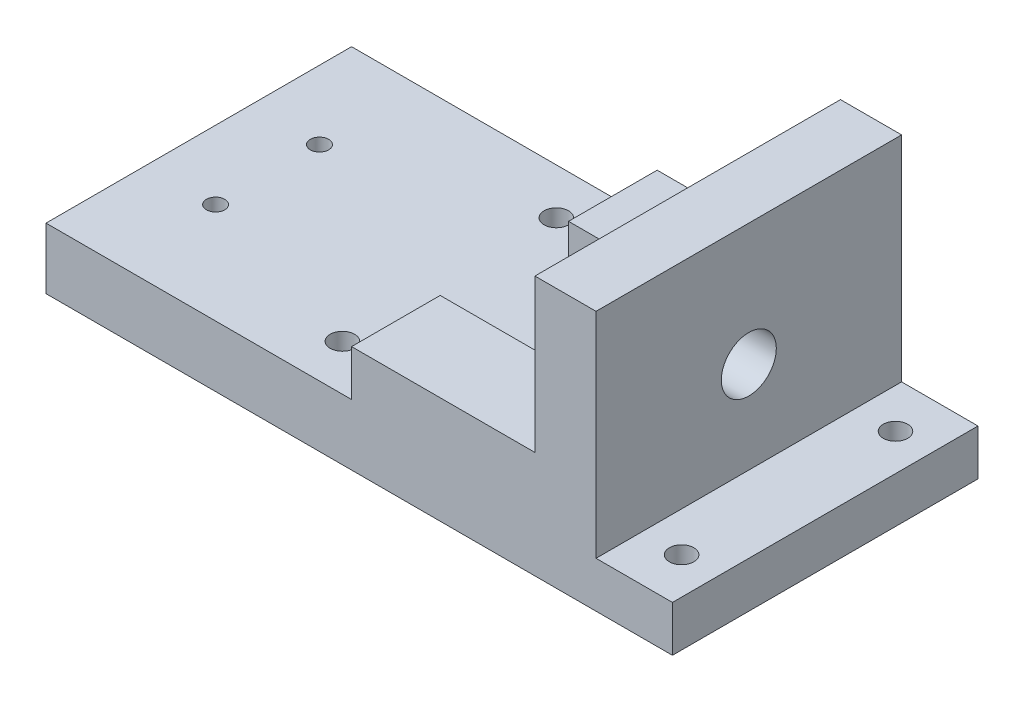
ISO-10303-21;
HEADER;
FILE_DESCRIPTION(('STEP AP214'),'2;1');
FILE_NAME('part.step','',(''),(''),'','','');
FILE_SCHEMA(('AUTOMOTIVE_DESIGN { 1 0 10303 214 1 1 1 1 }'));
ENDSEC;
DATA;
#1=APPLICATION_CONTEXT('core data for automotive mechanical design processes');
#2=APPLICATION_PROTOCOL_DEFINITION('international standard','automotive_design',2000,#1);
#3=PRODUCT_CONTEXT('',#1,'mechanical');
#4=PRODUCT('Part','Part','',(#3));
#5=PRODUCT_RELATED_PRODUCT_CATEGORY('part','',(#4));
#6=PRODUCT_DEFINITION_FORMATION('','',#4);
#7=PRODUCT_DEFINITION_CONTEXT('part definition',#1,'design');
#8=PRODUCT_DEFINITION('design','',#6,#7);
#9=PRODUCT_DEFINITION_SHAPE('','',#8);
#10=(LENGTH_UNIT() NAMED_UNIT(*) SI_UNIT(.MILLI.,.METRE.));
#11=(NAMED_UNIT(*) PLANE_ANGLE_UNIT() SI_UNIT($,.RADIAN.));
#12=(NAMED_UNIT(*) SI_UNIT($,.STERADIAN.) SOLID_ANGLE_UNIT());
#13=UNCERTAINTY_MEASURE_WITH_UNIT(LENGTH_MEASURE(1.E-05),#10,'distance_accuracy_value','');
#14=(GEOMETRIC_REPRESENTATION_CONTEXT(3) GLOBAL_UNCERTAINTY_ASSIGNED_CONTEXT((#13)) GLOBAL_UNIT_ASSIGNED_CONTEXT((#10,
#11,#12)) REPRESENTATION_CONTEXT('',''));
#15=CARTESIAN_POINT('',(0.,0.,0.));
#16=DIRECTION('',(0.,0.,1.));
#17=DIRECTION('',(1.,0.,0.));
#18=AXIS2_PLACEMENT_3D('',#15,#16,#17);
#19=CARTESIAN_POINT('',(-2.49999999999999,35.,50.));
#20=DIRECTION('',(0.,-1.,0.));
#21=DIRECTION('',(0.,0.,-1.));
#22=AXIS2_PLACEMENT_3D('',#19,#20,#21);
#23=PLANE('',#22);
#24=DIRECTION('',(0.,0.,-1.));
#25=VECTOR('',#24,1.);
#26=CARTESIAN_POINT('',(57.5,35.,50.));
#27=LINE('',#26,#25);
#28=CARTESIAN_POINT('',(57.5,35.,50.));
#29=VERTEX_POINT('',#28);
#30=CARTESIAN_POINT('',(57.5,35.,21.));
#31=VERTEX_POINT('',#30);
#32=EDGE_CURVE('E200',#29,#31,#27,.T.);
#33=ORIENTED_EDGE('',*,*,#32,.T.);
#34=DIRECTION('',(1.,0.,0.));
#35=VECTOR('',#34,1.);
#36=CARTESIAN_POINT('',(-2.49999999999998,35.,21.));
#37=LINE('',#36,#35);
#38=CARTESIAN_POINT('',(-2.49999999999998,35.,21.));
#39=VERTEX_POINT('',#38);
#40=EDGE_CURVE('E253',#39,#31,#37,.T.);
#41=ORIENTED_EDGE('',*,*,#40,.F.);
#42=DIRECTION('',(0.,0.,-1.));
#43=VECTOR('',#42,1.);
#44=CARTESIAN_POINT('',(-2.49999999999999,35.,50.));
#45=LINE('',#44,#43);
#46=CARTESIAN_POINT('',(-2.49999999999999,35.,50.));
#47=VERTEX_POINT('',#46);
#48=EDGE_CURVE('E198',#47,#39,#45,.T.);
#49=ORIENTED_EDGE('',*,*,#48,.F.);
#50=DIRECTION('',(-1.,0.,0.));
#51=VECTOR('',#50,1.);
#52=CARTESIAN_POINT('',(-2.49999999999999,35.,50.));
#53=LINE('',#52,#51);
#54=EDGE_CURVE('E144',#29,#47,#53,.T.);
#55=ORIENTED_EDGE('',*,*,#54,.F.);
#56=EDGE_LOOP('',(#33,#41,#49,#55));
#57=FACE_BOUND('',#56,.T.);
#58=ADVANCED_FACE('F41',(#57),#23,.F.);
#59=CARTESIAN_POINT('',(-2.49999999999999,20.,50.));
#60=DIRECTION('',(1.,0.,0.));
#61=DIRECTION('',(0.,0.,-1.));
#62=AXIS2_PLACEMENT_3D('',#59,#60,#61);
#63=PLANE('',#62);
#64=ORIENTED_EDGE('',*,*,#48,.T.);
#65=DIRECTION('',(0.,1.,0.));
#66=VECTOR('',#65,1.);
#67=CARTESIAN_POINT('',(-2.49999999999998,-53.2393336944022,21.));
#68=LINE('',#67,#66);
#69=CARTESIAN_POINT('',(-2.49999999999998,20.,21.));
#70=VERTEX_POINT('',#69);
#71=EDGE_CURVE('E156',#70,#39,#68,.T.);
#72=ORIENTED_EDGE('',*,*,#71,.F.);
#73=DIRECTION('',(0.,0.,-1.));
#74=VECTOR('',#73,1.);
#75=CARTESIAN_POINT('',(-2.49999999999999,20.,50.));
#76=LINE('',#75,#74);
#77=CARTESIAN_POINT('',(-2.49999999999999,20.,50.));
#78=VERTEX_POINT('',#77);
#79=EDGE_CURVE('E155',#78,#70,#76,.T.);
#80=ORIENTED_EDGE('',*,*,#79,.F.);
#81=DIRECTION('',(0.,-1.,0.));
#82=VECTOR('',#81,1.);
#83=CARTESIAN_POINT('',(-2.49999999999999,20.,50.));
#84=LINE('',#83,#82);
#85=EDGE_CURVE('E137',#47,#78,#84,.T.);
#86=ORIENTED_EDGE('',*,*,#85,.F.);
#87=EDGE_LOOP('',(#64,#72,#80,#86));
#88=FACE_BOUND('',#87,.T.);
#89=ADVANCED_FACE('F153',(#88),#63,.F.);
#90=CARTESIAN_POINT('',(102.5,15.,50.));
#91=DIRECTION('',(-1.,0.,0.));
#92=DIRECTION('',(0.,0.,1.));
#93=AXIS2_PLACEMENT_3D('',#90,#91,#92);
#94=PLANE('',#93);
#95=DIRECTION('',(0.,1.,0.));
#96=VECTOR('',#95,1.);
#97=CARTESIAN_POINT('',(102.5,15.,-50.));
#98=LINE('',#97,#96);
#99=CARTESIAN_POINT('',(102.5,0.,-50.));
#100=VERTEX_POINT('',#99);
#101=CARTESIAN_POINT('',(102.5,15.,-50.));
#102=VERTEX_POINT('',#101);
#103=EDGE_CURVE('E173',#100,#102,#98,.T.);
#104=ORIENTED_EDGE('',*,*,#103,.T.);
#105=DIRECTION('',(0.,0.,-1.));
#106=VECTOR('',#105,1.);
#107=CARTESIAN_POINT('',(102.5,15.,50.));
#108=LINE('',#107,#106);
#109=CARTESIAN_POINT('',(102.5,15.,50.));
#110=VERTEX_POINT('',#109);
#111=EDGE_CURVE('E49',#110,#102,#108,.T.);
#112=ORIENTED_EDGE('',*,*,#111,.F.);
#113=DIRECTION('',(0.,1.,0.));
#114=VECTOR('',#113,1.);
#115=CARTESIAN_POINT('',(102.5,15.,50.));
#116=LINE('',#115,#114);
#117=CARTESIAN_POINT('',(102.5,0.,50.));
#118=VERTEX_POINT('',#117);
#119=EDGE_CURVE('E113',#118,#110,#116,.T.);
#120=ORIENTED_EDGE('',*,*,#119,.F.);
#121=DIRECTION('',(0.,0.,-1.));
#122=VECTOR('',#121,1.);
#123=CARTESIAN_POINT('',(102.5,0.,50.));
#124=LINE('',#123,#122);
#125=EDGE_CURVE('E11',#118,#100,#124,.T.);
#126=ORIENTED_EDGE('',*,*,#125,.T.);
#127=EDGE_LOOP('',(#104,#112,#120,#126));
#128=FACE_BOUND('',#127,.T.);
#129=ADVANCED_FACE('F43',(#128),#94,.F.);
#130=CARTESIAN_POINT('',(77.5,15.,50.));
#131=DIRECTION('',(0.,-1.,0.));
#132=DIRECTION('',(1.,0.,0.));
#133=AXIS2_PLACEMENT_3D('',#130,#131,#132);
#134=PLANE('',#133);
#135=CARTESIAN_POINT('',(90.5,15.,-35.));
#136=DIRECTION('',(0.,1.,0.));
#137=DIRECTION('',(-1.,0.,0.));
#138=AXIS2_PLACEMENT_3D('',#135,#136,#137);
#139=CIRCLE('',#138,4.00000000000001);
#140=CARTESIAN_POINT('',(86.5,15.,-35.));
#141=VERTEX_POINT('',#140);
#142=EDGE_CURVE('E216',#141,#141,#139,.T.);
#143=ORIENTED_EDGE('',*,*,#142,.F.);
#144=EDGE_LOOP('',(#143));
#145=FACE_BOUND('',#144,.T.);
#146=CARTESIAN_POINT('',(90.5,15.,35.));
#147=DIRECTION('',(0.,1.,0.));
#148=DIRECTION('',(1.,0.,0.));
#149=AXIS2_PLACEMENT_3D('',#146,#147,#148);
#150=CIRCLE('',#149,4.00000000000001);
#151=CARTESIAN_POINT('',(94.5,15.,35.));
#152=VERTEX_POINT('',#151);
#153=EDGE_CURVE('E269',#152,#152,#150,.T.);
#154=ORIENTED_EDGE('',*,*,#153,.F.);
#155=EDGE_LOOP('',(#154));
#156=FACE_BOUND('',#155,.T.);
#157=DIRECTION('',(-1.,0.,0.));
#158=VECTOR('',#157,1.);
#159=CARTESIAN_POINT('',(77.5,15.,-50.));
#160=LINE('',#159,#158);
#161=CARTESIAN_POINT('',(77.5,15.,-50.));
#162=VERTEX_POINT('',#161);
#163=EDGE_CURVE('E171',#102,#162,#160,.T.);
#164=ORIENTED_EDGE('',*,*,#163,.T.);
#165=DIRECTION('',(0.,0.,-1.));
#166=VECTOR('',#165,1.);
#167=CARTESIAN_POINT('',(77.5,15.,50.));
#168=LINE('',#167,#166);
#169=CARTESIAN_POINT('',(77.5,15.,50.));
#170=VERTEX_POINT('',#169);
#171=EDGE_CURVE('E208',#170,#162,#168,.T.);
#172=ORIENTED_EDGE('',*,*,#171,.F.);
#173=DIRECTION('',(-1.,0.,0.));
#174=VECTOR('',#173,1.);
#175=CARTESIAN_POINT('',(77.5,15.,50.));
#176=LINE('',#175,#174);
#177=EDGE_CURVE('E280',#110,#170,#176,.T.);
#178=ORIENTED_EDGE('',*,*,#177,.F.);
#179=ORIENTED_EDGE('',*,*,#111,.T.);
#180=EDGE_LOOP('',(#164,#172,#178,#179));
#181=FACE_BOUND('',#180,.T.);
#182=ADVANCED_FACE('F352',(#145,#156,#181),#134,.F.);
#183=CARTESIAN_POINT('',(77.5,85.,50.));
#184=DIRECTION('',(-1.,0.,0.));
#185=DIRECTION('',(0.,-1.,0.));
#186=AXIS2_PLACEMENT_3D('',#183,#184,#185);
#187=PLANE('',#186);
#188=CARTESIAN_POINT('',(77.5,45.,0.));
#189=DIRECTION('',(1.,0.,0.));
#190=DIRECTION('',(0.,1.,0.));
#191=AXIS2_PLACEMENT_3D('',#188,#189,#190);
#192=CIRCLE('',#191,9.);
#193=CARTESIAN_POINT('',(77.5,54.,0.));
#194=VERTEX_POINT('',#193);
#195=EDGE_CURVE('E224',#194,#194,#192,.T.);
#196=ORIENTED_EDGE('',*,*,#195,.F.);
#197=EDGE_LOOP('',(#196));
#198=FACE_BOUND('',#197,.T.);
#199=DIRECTION('',(0.,1.,0.));
#200=VECTOR('',#199,1.);
#201=CARTESIAN_POINT('',(77.5,85.,-50.));
#202=LINE('',#201,#200);
#203=CARTESIAN_POINT('',(77.5,85.,-50.));
#204=VERTEX_POINT('',#203);
#205=EDGE_CURVE('E178',#162,#204,#202,.T.);
#206=ORIENTED_EDGE('',*,*,#205,.T.);
#207=DIRECTION('',(0.,0.,-1.));
#208=VECTOR('',#207,1.);
#209=CARTESIAN_POINT('',(77.5,85.,50.));
#210=LINE('',#209,#208);
#211=CARTESIAN_POINT('',(77.5,85.,50.));
#212=VERTEX_POINT('',#211);
#213=EDGE_CURVE('E202',#212,#204,#210,.T.);
#214=ORIENTED_EDGE('',*,*,#213,.F.);
#215=DIRECTION('',(0.,1.,0.));
#216=VECTOR('',#215,1.);
#217=CARTESIAN_POINT('',(77.5,85.,50.));
#218=LINE('',#217,#216);
#219=EDGE_CURVE('E276',#170,#212,#218,.T.);
#220=ORIENTED_EDGE('',*,*,#219,.F.);
#221=ORIENTED_EDGE('',*,*,#171,.T.);
#222=EDGE_LOOP('',(#206,#214,#220,#221));
#223=FACE_BOUND('',#222,.T.);
#224=ADVANCED_FACE('F363',(#198,#223),#187,.F.);
#225=CARTESIAN_POINT('',(57.5,85.,50.));
#226=DIRECTION('',(0.,-1.,0.));
#227=DIRECTION('',(0.,0.,-1.));
#228=AXIS2_PLACEMENT_3D('',#225,#226,#227);
#229=PLANE('',#228);
#230=DIRECTION('',(-1.,0.,0.));
#231=VECTOR('',#230,1.);
#232=CARTESIAN_POINT('',(57.5,85.,-50.));
#233=LINE('',#232,#231);
#234=CARTESIAN_POINT('',(57.5,85.,-50.));
#235=VERTEX_POINT('',#234);
#236=EDGE_CURVE('E177',#204,#235,#233,.T.);
#237=ORIENTED_EDGE('',*,*,#236,.T.);
#238=DIRECTION('',(0.,0.,-1.));
#239=VECTOR('',#238,1.);
#240=CARTESIAN_POINT('',(57.5,85.,50.));
#241=LINE('',#240,#239);
#242=CARTESIAN_POINT('',(57.5,85.,50.));
#243=VERTEX_POINT('',#242);
#244=EDGE_CURVE('E205',#243,#235,#241,.T.);
#245=ORIENTED_EDGE('',*,*,#244,.F.);
#246=DIRECTION('',(-1.,0.,0.));
#247=VECTOR('',#246,1.);
#248=CARTESIAN_POINT('',(57.5,85.,50.));
#249=LINE('',#248,#247);
#250=EDGE_CURVE('E283',#212,#243,#249,.T.);
#251=ORIENTED_EDGE('',*,*,#250,.F.);
#252=ORIENTED_EDGE('',*,*,#213,.T.);
#253=EDGE_LOOP('',(#237,#245,#251,#252));
#254=FACE_BOUND('',#253,.T.);
#255=ADVANCED_FACE('F340',(#254),#229,.F.);
#256=CARTESIAN_POINT('',(57.5,35.,50.));
#257=DIRECTION('',(1.,0.,0.));
#258=DIRECTION('',(0.,0.,-1.));
#259=AXIS2_PLACEMENT_3D('',#256,#257,#258);
#260=PLANE('',#259);
#261=CARTESIAN_POINT('',(57.5,45.,0.));
#262=DIRECTION('',(1.,0.,0.));
#263=DIRECTION('',(0.,0.,-1.));
#264=AXIS2_PLACEMENT_3D('',#261,#262,#263);
#265=CIRCLE('',#264,9.);
#266=CARTESIAN_POINT('',(57.5,45.,-9.));
#267=VERTEX_POINT('',#266);
#268=EDGE_CURVE('E218',#267,#267,#265,.T.);
#269=ORIENTED_EDGE('',*,*,#268,.T.);
#270=EDGE_LOOP('',(#269));
#271=FACE_BOUND('',#270,.T.);
#272=DIRECTION('',(0.,-1.,0.));
#273=VECTOR('',#272,1.);
#274=CARTESIAN_POINT('',(57.5,35.,-50.));
#275=LINE('',#274,#273);
#276=CARTESIAN_POINT('',(57.5,35.,-50.));
#277=VERTEX_POINT('',#276);
#278=EDGE_CURVE('E176',#235,#277,#275,.T.);
#279=ORIENTED_EDGE('',*,*,#278,.T.);
#280=CARTESIAN_POINT('',(57.5,35.,-21.));
#281=VERTEX_POINT('',#280);
#282=EDGE_CURVE('E196',#281,#277,#27,.T.);
#283=ORIENTED_EDGE('',*,*,#282,.F.);
#284=DIRECTION('',(0.,1.,0.));
#285=VECTOR('',#284,1.);
#286=CARTESIAN_POINT('',(57.5,-53.2393336944022,-21.));
#287=LINE('',#286,#285);
#288=CARTESIAN_POINT('',(57.5,20.,-21.));
#289=VERTEX_POINT('',#288);
#290=EDGE_CURVE('E260',#289,#281,#287,.T.);
#291=ORIENTED_EDGE('',*,*,#290,.F.);
#292=DIRECTION('',(0.,0.,-1.));
#293=VECTOR('',#292,1.);
#294=CARTESIAN_POINT('',(57.5,20.,21.));
#295=LINE('',#294,#293);
#296=CARTESIAN_POINT('',(57.5,20.,21.));
#297=VERTEX_POINT('',#296);
#298=EDGE_CURVE('E256',#297,#289,#295,.T.);
#299=ORIENTED_EDGE('',*,*,#298,.F.);
#300=DIRECTION('',(0.,1.,0.));
#301=VECTOR('',#300,1.);
#302=CARTESIAN_POINT('',(57.5,-53.2393336944022,21.));
#303=LINE('',#302,#301);
#304=EDGE_CURVE('E261',#297,#31,#303,.T.);
#305=ORIENTED_EDGE('',*,*,#304,.T.);
#306=ORIENTED_EDGE('',*,*,#32,.F.);
#307=DIRECTION('',(0.,-1.,0.));
#308=VECTOR('',#307,1.);
#309=CARTESIAN_POINT('',(57.5,35.,50.));
#310=LINE('',#309,#308);
#311=EDGE_CURVE('E281',#243,#29,#310,.T.);
#312=ORIENTED_EDGE('',*,*,#311,.F.);
#313=ORIENTED_EDGE('',*,*,#244,.T.);
#314=EDGE_LOOP('',(#279,#283,#291,#299,#305,#306,#312,#313));
#315=FACE_BOUND('',#314,.T.);
#316=ADVANCED_FACE('F290',(#271,#315),#260,.F.);
#317=CARTESIAN_POINT('',(-2.49999999999999,35.,-21.));
#318=VERTEX_POINT('',#317);
#319=CARTESIAN_POINT('',(-2.49999999999999,35.,-50.));
#320=VERTEX_POINT('',#319);
#321=EDGE_CURVE('E157',#318,#320,#45,.T.);
#322=ORIENTED_EDGE('',*,*,#321,.F.);
#323=DIRECTION('',(-1.,0.,0.));
#324=VECTOR('',#323,1.);
#325=CARTESIAN_POINT('',(57.5,35.,-21.));
#326=LINE('',#325,#324);
#327=EDGE_CURVE('E225',#281,#318,#326,.T.);
#328=ORIENTED_EDGE('',*,*,#327,.F.);
#329=ORIENTED_EDGE('',*,*,#282,.T.);
#330=DIRECTION('',(-1.,0.,0.));
#331=VECTOR('',#330,1.);
#332=CARTESIAN_POINT('',(-2.49999999999999,35.,-50.));
#333=LINE('',#332,#331);
#334=EDGE_CURVE('E181',#277,#320,#333,.T.);
#335=ORIENTED_EDGE('',*,*,#334,.T.);
#336=EDGE_LOOP('',(#322,#328,#329,#335));
#337=FACE_BOUND('',#336,.T.);
#338=ADVANCED_FACE('F322',(#337),#23,.F.);
#339=CARTESIAN_POINT('',(-2.49999999999999,20.,-21.));
#340=VERTEX_POINT('',#339);
#341=CARTESIAN_POINT('',(-2.49999999999999,20.,-50.));
#342=VERTEX_POINT('',#341);
#343=EDGE_CURVE('E159',#340,#342,#76,.T.);
#344=ORIENTED_EDGE('',*,*,#343,.F.);
#345=DIRECTION('',(0.,1.,0.));
#346=VECTOR('',#345,1.);
#347=CARTESIAN_POINT('',(-2.49999999999999,-53.2393336944022,-21.));
#348=LINE('',#347,#346);
#349=EDGE_CURVE('E59',#340,#318,#348,.T.);
#350=ORIENTED_EDGE('',*,*,#349,.T.);
#351=ORIENTED_EDGE('',*,*,#321,.T.);
#352=DIRECTION('',(0.,-1.,0.));
#353=VECTOR('',#352,1.);
#354=CARTESIAN_POINT('',(-2.49999999999999,20.,-50.));
#355=LINE('',#354,#353);
#356=EDGE_CURVE('E188',#320,#342,#355,.T.);
#357=ORIENTED_EDGE('',*,*,#356,.T.);
#358=EDGE_LOOP('',(#344,#350,#351,#357));
#359=FACE_BOUND('',#358,.T.);
#360=ADVANCED_FACE('F328',(#359),#63,.F.);
#361=CARTESIAN_POINT('',(-102.5,20.,50.));
#362=DIRECTION('',(0.,-1.,0.));
#363=DIRECTION('',(1.,0.,0.));
#364=AXIS2_PLACEMENT_3D('',#361,#362,#363);
#365=PLANE('',#364);
#366=CARTESIAN_POINT('',(-80.,20.,17.));
#367=DIRECTION('',(0.,1.,0.));
#368=DIRECTION('',(-1.,0.,0.));
#369=AXIS2_PLACEMENT_3D('',#366,#367,#368);
#370=CIRCLE('',#369,3.00000000000001);
#371=CARTESIAN_POINT('',(-83.,20.,17.));
#372=VERTEX_POINT('',#371);
#373=EDGE_CURVE('E234',#372,#372,#370,.T.);
#374=ORIENTED_EDGE('',*,*,#373,.F.);
#375=EDGE_LOOP('',(#374));
#376=FACE_BOUND('',#375,.T.);
#377=CARTESIAN_POINT('',(-79.9999999999999,20.,-17.));
#378=DIRECTION('',(0.,1.,0.));
#379=DIRECTION('',(1.,0.,0.));
#380=AXIS2_PLACEMENT_3D('',#377,#378,#379);
#381=CIRCLE('',#380,3.00000000000001);
#382=CARTESIAN_POINT('',(-76.9999999999999,20.,-17.));
#383=VERTEX_POINT('',#382);
#384=EDGE_CURVE('E236',#383,#383,#381,.T.);
#385=ORIENTED_EDGE('',*,*,#384,.F.);
#386=EDGE_LOOP('',(#385));
#387=FACE_BOUND('',#386,.T.);
#388=CARTESIAN_POINT('',(-20.5,20.,35.));
#389=DIRECTION('',(0.,1.,0.));
#390=DIRECTION('',(-1.,0.,0.));
#391=AXIS2_PLACEMENT_3D('',#388,#389,#390);
#392=CIRCLE('',#391,4.);
#393=CARTESIAN_POINT('',(-24.5,20.,35.));
#394=VERTEX_POINT('',#393);
#395=EDGE_CURVE('E226',#394,#394,#392,.T.);
#396=ORIENTED_EDGE('',*,*,#395,.F.);
#397=EDGE_LOOP('',(#396));
#398=FACE_BOUND('',#397,.T.);
#399=CARTESIAN_POINT('',(-20.5,20.,-35.));
#400=DIRECTION('',(0.,1.,0.));
#401=DIRECTION('',(1.,0.,0.));
#402=AXIS2_PLACEMENT_3D('',#399,#400,#401);
#403=CIRCLE('',#402,4.);
#404=CARTESIAN_POINT('',(-16.5,20.,-35.));
#405=VERTEX_POINT('',#404);
#406=EDGE_CURVE('E237',#405,#405,#403,.T.);
#407=ORIENTED_EDGE('',*,*,#406,.F.);
#408=EDGE_LOOP('',(#407));
#409=FACE_BOUND('',#408,.T.);
#410=DIRECTION('',(-1.,0.,0.));
#411=VECTOR('',#410,1.);
#412=CARTESIAN_POINT('',(-102.5,20.,-50.));
#413=LINE('',#412,#411);
#414=CARTESIAN_POINT('',(-102.5,20.,-50.));
#415=VERTEX_POINT('',#414);
#416=EDGE_CURVE('E187',#342,#415,#413,.T.);
#417=ORIENTED_EDGE('',*,*,#416,.T.);
#418=DIRECTION('',(0.,0.,-1.));
#419=VECTOR('',#418,1.);
#420=CARTESIAN_POINT('',(-102.5,20.,50.));
#421=LINE('',#420,#419);
#422=CARTESIAN_POINT('',(-102.5,20.,50.));
#423=VERTEX_POINT('',#422);
#424=EDGE_CURVE('E162',#423,#415,#421,.T.);
#425=ORIENTED_EDGE('',*,*,#424,.F.);
#426=DIRECTION('',(-1.,0.,0.));
#427=VECTOR('',#426,1.);
#428=CARTESIAN_POINT('',(-102.5,20.,50.));
#429=LINE('',#428,#427);
#430=EDGE_CURVE('E142',#78,#423,#429,.T.);
#431=ORIENTED_EDGE('',*,*,#430,.F.);
#432=ORIENTED_EDGE('',*,*,#79,.T.);
#433=DIRECTION('',(1.,0.,0.));
#434=VECTOR('',#433,1.);
#435=CARTESIAN_POINT('',(-2.49999999999999,20.,21.));
#436=LINE('',#435,#434);
#437=EDGE_CURVE('E265',#70,#297,#436,.T.);
#438=ORIENTED_EDGE('',*,*,#437,.T.);
#439=ORIENTED_EDGE('',*,*,#298,.T.);
#440=DIRECTION('',(-1.,0.,0.));
#441=VECTOR('',#440,1.);
#442=CARTESIAN_POINT('',(57.5,20.,-21.));
#443=LINE('',#442,#441);
#444=EDGE_CURVE('E254',#289,#340,#443,.T.);
#445=ORIENTED_EDGE('',*,*,#444,.T.);
#446=ORIENTED_EDGE('',*,*,#343,.T.);
#447=EDGE_LOOP('',(#417,#425,#431,#432,#438,#439,#445,#446));
#448=FACE_BOUND('',#447,.T.);
#449=ADVANCED_FACE('F165',(#376,#387,#398,#409,#448),#365,.F.);
#450=CARTESIAN_POINT('',(-102.5,0.,50.));
#451=DIRECTION('',(1.,0.,0.));
#452=DIRECTION('',(0.,0.,-1.));
#453=AXIS2_PLACEMENT_3D('',#450,#451,#452);
#454=PLANE('',#453);
#455=DIRECTION('',(0.,-1.,0.));
#456=VECTOR('',#455,1.);
#457=CARTESIAN_POINT('',(-102.5,0.,-50.));
#458=LINE('',#457,#456);
#459=CARTESIAN_POINT('',(-102.5,0.,-50.));
#460=VERTEX_POINT('',#459);
#461=EDGE_CURVE('E107',#415,#460,#458,.T.);
#462=ORIENTED_EDGE('',*,*,#461,.T.);
#463=DIRECTION('',(0.,0.,-1.));
#464=VECTOR('',#463,1.);
#465=CARTESIAN_POINT('',(-102.5,0.,50.));
#466=LINE('',#465,#464);
#467=CARTESIAN_POINT('',(-102.5,0.,50.));
#468=VERTEX_POINT('',#467);
#469=EDGE_CURVE('E170',#468,#460,#466,.T.);
#470=ORIENTED_EDGE('',*,*,#469,.F.);
#471=DIRECTION('',(0.,-1.,0.));
#472=VECTOR('',#471,1.);
#473=CARTESIAN_POINT('',(-102.5,0.,50.));
#474=LINE('',#473,#472);
#475=EDGE_CURVE('E164',#423,#468,#474,.T.);
#476=ORIENTED_EDGE('',*,*,#475,.F.);
#477=ORIENTED_EDGE('',*,*,#424,.T.);
#478=EDGE_LOOP('',(#462,#470,#476,#477));
#479=FACE_BOUND('',#478,.T.);
#480=ADVANCED_FACE('F347',(#479),#454,.F.);
#481=CARTESIAN_POINT('',(0.,0.,50.));
#482=DIRECTION('',(0.,1.,0.));
#483=DIRECTION('',(-1.,0.,0.));
#484=AXIS2_PLACEMENT_3D('',#481,#482,#483);
#485=PLANE('',#484);
#486=CARTESIAN_POINT('',(-80.,0.,17.));
#487=DIRECTION('',(0.,1.,0.));
#488=DIRECTION('',(-1.,0.,0.));
#489=AXIS2_PLACEMENT_3D('',#486,#487,#488);
#490=CIRCLE('',#489,3.00000000000001);
#491=CARTESIAN_POINT('',(-83.,0.,17.));
#492=VERTEX_POINT('',#491);
#493=EDGE_CURVE('E44',#492,#492,#490,.T.);
#494=ORIENTED_EDGE('',*,*,#493,.T.);
#495=EDGE_LOOP('',(#494));
#496=FACE_BOUND('',#495,.T.);
#497=CARTESIAN_POINT('',(-79.9999999999999,0.,-17.));
#498=DIRECTION('',(0.,1.,0.));
#499=DIRECTION('',(-1.,0.,0.));
#500=AXIS2_PLACEMENT_3D('',#497,#498,#499);
#501=CIRCLE('',#500,3.00000000000001);
#502=CARTESIAN_POINT('',(-82.9999999999999,0.,-17.));
#503=VERTEX_POINT('',#502);
#504=EDGE_CURVE('E229',#503,#503,#501,.T.);
#505=ORIENTED_EDGE('',*,*,#504,.T.);
#506=EDGE_LOOP('',(#505));
#507=FACE_BOUND('',#506,.T.);
#508=CARTESIAN_POINT('',(-20.5,0.,35.));
#509=DIRECTION('',(0.,1.,0.));
#510=DIRECTION('',(-1.,0.,0.));
#511=AXIS2_PLACEMENT_3D('',#508,#509,#510);
#512=CIRCLE('',#511,4.);
#513=CARTESIAN_POINT('',(-24.5,0.,35.));
#514=VERTEX_POINT('',#513);
#515=EDGE_CURVE('E230',#514,#514,#512,.T.);
#516=ORIENTED_EDGE('',*,*,#515,.T.);
#517=EDGE_LOOP('',(#516));
#518=FACE_BOUND('',#517,.T.);
#519=CARTESIAN_POINT('',(-20.5,0.,-35.));
#520=DIRECTION('',(0.,1.,0.));
#521=DIRECTION('',(-1.,0.,0.));
#522=AXIS2_PLACEMENT_3D('',#519,#520,#521);
#523=CIRCLE('',#522,4.);
#524=CARTESIAN_POINT('',(-24.5,0.,-35.));
#525=VERTEX_POINT('',#524);
#526=EDGE_CURVE('E221',#525,#525,#523,.T.);
#527=ORIENTED_EDGE('',*,*,#526,.T.);
#528=EDGE_LOOP('',(#527));
#529=FACE_BOUND('',#528,.T.);
#530=CARTESIAN_POINT('',(90.5,0.,-35.));
#531=DIRECTION('',(0.,1.,0.));
#532=DIRECTION('',(-1.,0.,0.));
#533=AXIS2_PLACEMENT_3D('',#530,#531,#532);
#534=CIRCLE('',#533,4.00000000000001);
#535=CARTESIAN_POINT('',(86.5,0.,-35.));
#536=VERTEX_POINT('',#535);
#537=EDGE_CURVE('E172',#536,#536,#534,.T.);
#538=ORIENTED_EDGE('',*,*,#537,.T.);
#539=EDGE_LOOP('',(#538));
#540=FACE_BOUND('',#539,.T.);
#541=CARTESIAN_POINT('',(90.5,0.,35.));
#542=DIRECTION('',(0.,1.,0.));
#543=DIRECTION('',(-1.,0.,0.));
#544=AXIS2_PLACEMENT_3D('',#541,#542,#543);
#545=CIRCLE('',#544,4.00000000000001);
#546=CARTESIAN_POINT('',(86.5,0.,35.));
#547=VERTEX_POINT('',#546);
#548=EDGE_CURVE('E213',#547,#547,#545,.T.);
#549=ORIENTED_EDGE('',*,*,#548,.T.);
#550=EDGE_LOOP('',(#549));
#551=FACE_BOUND('',#550,.T.);
#552=DIRECTION('',(1.,0.,0.));
#553=VECTOR('',#552,1.);
#554=CARTESIAN_POINT('',(0.,0.,-50.));
#555=LINE('',#554,#553);
#556=EDGE_CURVE('E194',#460,#100,#555,.T.);
#557=ORIENTED_EDGE('',*,*,#556,.T.);
#558=ORIENTED_EDGE('',*,*,#125,.F.);
#559=DIRECTION('',(1.,0.,0.));
#560=VECTOR('',#559,1.);
#561=CARTESIAN_POINT('',(102.5,0.,50.));
#562=LINE('',#561,#560);
#563=EDGE_CURVE('E69',#468,#118,#562,.T.);
#564=ORIENTED_EDGE('',*,*,#563,.F.);
#565=ORIENTED_EDGE('',*,*,#469,.T.);
#566=EDGE_LOOP('',(#557,#558,#564,#565));
#567=FACE_BOUND('',#566,.T.);
#568=ADVANCED_FACE('F353',(#496,#507,#518,#529,#540,#551,#567),#485,.F.);
#569=CARTESIAN_POINT('',(0.,0.,50.));
#570=DIRECTION('',(0.,0.,-1.));
#571=DIRECTION('',(-1.,0.,0.));
#572=AXIS2_PLACEMENT_3D('',#569,#570,#571);
#573=PLANE('',#572);
#574=ORIENTED_EDGE('',*,*,#563,.T.);
#575=ORIENTED_EDGE('',*,*,#119,.T.);
#576=ORIENTED_EDGE('',*,*,#177,.T.);
#577=ORIENTED_EDGE('',*,*,#219,.T.);
#578=ORIENTED_EDGE('',*,*,#250,.T.);
#579=ORIENTED_EDGE('',*,*,#311,.T.);
#580=ORIENTED_EDGE('',*,*,#54,.T.);
#581=ORIENTED_EDGE('',*,*,#85,.T.);
#582=ORIENTED_EDGE('',*,*,#430,.T.);
#583=ORIENTED_EDGE('',*,*,#475,.T.);
#584=EDGE_LOOP('',(#574,#575,#576,#577,#578,#579,#580,#581,#582,#583));
#585=FACE_BOUND('',#584,.T.);
#586=ADVANCED_FACE('F136',(#585),#573,.F.);
#587=CARTESIAN_POINT('',(0.,0.,-50.));
#588=DIRECTION('',(0.,0.,-1.));
#589=DIRECTION('',(-1.,0.,0.));
#590=AXIS2_PLACEMENT_3D('',#587,#588,#589);
#591=PLANE('',#590);
#592=ORIENTED_EDGE('',*,*,#103,.F.);
#593=ORIENTED_EDGE('',*,*,#556,.F.);
#594=ORIENTED_EDGE('',*,*,#461,.F.);
#595=ORIENTED_EDGE('',*,*,#416,.F.);
#596=ORIENTED_EDGE('',*,*,#356,.F.);
#597=ORIENTED_EDGE('',*,*,#334,.F.);
#598=ORIENTED_EDGE('',*,*,#278,.F.);
#599=ORIENTED_EDGE('',*,*,#236,.F.);
#600=ORIENTED_EDGE('',*,*,#205,.F.);
#601=ORIENTED_EDGE('',*,*,#163,.F.);
#602=EDGE_LOOP('',(#592,#593,#594,#595,#596,#597,#598,#599,#600,#601));
#603=FACE_BOUND('',#602,.T.);
#604=ADVANCED_FACE('F349',(#603),#591,.T.);
#605=CARTESIAN_POINT('',(90.5,-85.,35.));
#606=DIRECTION('',(0.,1.,0.));
#607=DIRECTION('',(-1.,0.,0.));
#608=AXIS2_PLACEMENT_3D('',#605,#606,#607);
#609=CYLINDRICAL_SURFACE('',#608,4.00000000000001);
#610=ORIENTED_EDGE('',*,*,#153,.T.);
#611=EDGE_LOOP('',(#610));
#612=FACE_BOUND('',#611,.T.);
#613=ORIENTED_EDGE('',*,*,#548,.F.);
#614=EDGE_LOOP('',(#613));
#615=FACE_BOUND('',#614,.T.);
#616=ADVANCED_FACE('F317',(#612,#615),#609,.F.);
#617=CARTESIAN_POINT('',(90.5,-85.,-35.));
#618=DIRECTION('',(0.,1.,0.));
#619=DIRECTION('',(-1.,0.,0.));
#620=AXIS2_PLACEMENT_3D('',#617,#618,#619);
#621=CYLINDRICAL_SURFACE('',#620,4.00000000000001);
#622=ORIENTED_EDGE('',*,*,#142,.T.);
#623=EDGE_LOOP('',(#622));
#624=FACE_BOUND('',#623,.T.);
#625=ORIENTED_EDGE('',*,*,#537,.F.);
#626=EDGE_LOOP('',(#625));
#627=FACE_BOUND('',#626,.T.);
#628=ADVANCED_FACE('F309',(#624,#627),#621,.F.);
#629=CARTESIAN_POINT('',(-2.49999999999998,-53.2393336944022,21.));
#630=DIRECTION('',(0.,0.,1.));
#631=DIRECTION('',(1.,0.,0.));
#632=AXIS2_PLACEMENT_3D('',#629,#630,#631);
#633=PLANE('',#632);
#634=ORIENTED_EDGE('',*,*,#71,.T.);
#635=ORIENTED_EDGE('',*,*,#40,.T.);
#636=ORIENTED_EDGE('',*,*,#304,.F.);
#637=ORIENTED_EDGE('',*,*,#437,.F.);
#638=EDGE_LOOP('',(#634,#635,#636,#637));
#639=FACE_BOUND('',#638,.T.);
#640=ADVANCED_FACE('F307',(#639),#633,.F.);
#641=CARTESIAN_POINT('',(57.5,-53.2393336944022,-21.));
#642=DIRECTION('',(0.,0.,-1.));
#643=DIRECTION('',(-1.,0.,0.));
#644=AXIS2_PLACEMENT_3D('',#641,#642,#643);
#645=PLANE('',#644);
#646=ORIENTED_EDGE('',*,*,#290,.T.);
#647=ORIENTED_EDGE('',*,*,#327,.T.);
#648=ORIENTED_EDGE('',*,*,#349,.F.);
#649=ORIENTED_EDGE('',*,*,#444,.F.);
#650=EDGE_LOOP('',(#646,#647,#648,#649));
#651=FACE_BOUND('',#650,.T.);
#652=ADVANCED_FACE('F310',(#651),#645,.F.);
#653=CARTESIAN_POINT('',(-22.5,45.,0.));
#654=DIRECTION('',(1.,0.,0.));
#655=DIRECTION('',(0.,0.,-1.));
#656=AXIS2_PLACEMENT_3D('',#653,#654,#655);
#657=CYLINDRICAL_SURFACE('',#656,9.);
#658=ORIENTED_EDGE('',*,*,#195,.T.);
#659=EDGE_LOOP('',(#658));
#660=FACE_BOUND('',#659,.T.);
#661=ORIENTED_EDGE('',*,*,#268,.F.);
#662=EDGE_LOOP('',(#661));
#663=FACE_BOUND('',#662,.T.);
#664=ADVANCED_FACE('F316',(#660,#663),#657,.F.);
#665=CARTESIAN_POINT('',(-20.5,-80.,-35.));
#666=DIRECTION('',(0.,1.,0.));
#667=DIRECTION('',(-1.,0.,0.));
#668=AXIS2_PLACEMENT_3D('',#665,#666,#667);
#669=CYLINDRICAL_SURFACE('',#668,4.);
#670=ORIENTED_EDGE('',*,*,#406,.T.);
#671=EDGE_LOOP('',(#670));
#672=FACE_BOUND('',#671,.T.);
#673=ORIENTED_EDGE('',*,*,#526,.F.);
#674=EDGE_LOOP('',(#673));
#675=FACE_BOUND('',#674,.T.);
#676=ADVANCED_FACE('F409',(#672,#675),#669,.F.);
#677=CARTESIAN_POINT('',(-20.5,-80.,35.));
#678=DIRECTION('',(0.,1.,0.));
#679=DIRECTION('',(-1.,0.,0.));
#680=AXIS2_PLACEMENT_3D('',#677,#678,#679);
#681=CYLINDRICAL_SURFACE('',#680,4.);
#682=ORIENTED_EDGE('',*,*,#395,.T.);
#683=EDGE_LOOP('',(#682));
#684=FACE_BOUND('',#683,.T.);
#685=ORIENTED_EDGE('',*,*,#515,.F.);
#686=EDGE_LOOP('',(#685));
#687=FACE_BOUND('',#686,.T.);
#688=ADVANCED_FACE('F412',(#684,#687),#681,.F.);
#689=CARTESIAN_POINT('',(-79.9999999999999,-80.,-17.));
#690=DIRECTION('',(0.,1.,0.));
#691=DIRECTION('',(-1.,0.,0.));
#692=AXIS2_PLACEMENT_3D('',#689,#690,#691);
#693=CYLINDRICAL_SURFACE('',#692,3.00000000000001);
#694=ORIENTED_EDGE('',*,*,#384,.T.);
#695=EDGE_LOOP('',(#694));
#696=FACE_BOUND('',#695,.T.);
#697=ORIENTED_EDGE('',*,*,#504,.F.);
#698=EDGE_LOOP('',(#697));
#699=FACE_BOUND('',#698,.T.);
#700=ADVANCED_FACE('F421',(#696,#699),#693,.F.);
#701=CARTESIAN_POINT('',(-80.,-80.,17.));
#702=DIRECTION('',(0.,1.,0.));
#703=DIRECTION('',(-1.,0.,0.));
#704=AXIS2_PLACEMENT_3D('',#701,#702,#703);
#705=CYLINDRICAL_SURFACE('',#704,3.00000000000001);
#706=ORIENTED_EDGE('',*,*,#373,.T.);
#707=EDGE_LOOP('',(#706));
#708=FACE_BOUND('',#707,.T.);
#709=ORIENTED_EDGE('',*,*,#493,.F.);
#710=EDGE_LOOP('',(#709));
#711=FACE_BOUND('',#710,.T.);
#712=ADVANCED_FACE('F429',(#708,#711),#705,.F.);
#713=CLOSED_SHELL('',(#58,#89,#129,#182,#224,#255,#316,#338,#360,#449,#480,#568,#586,#604,#616,
#628,#640,#652,#664,#676,#688,#700,#712));
#714=MANIFOLD_SOLID_BREP('B2',#713);
#715=ADVANCED_BREP_SHAPE_REPRESENTATION('',(#18,#714),#14);
#716=SHAPE_DEFINITION_REPRESENTATION(#9,#715);
ENDSEC;
END-ISO-10303-21;
